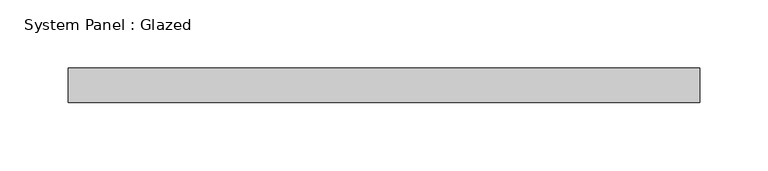
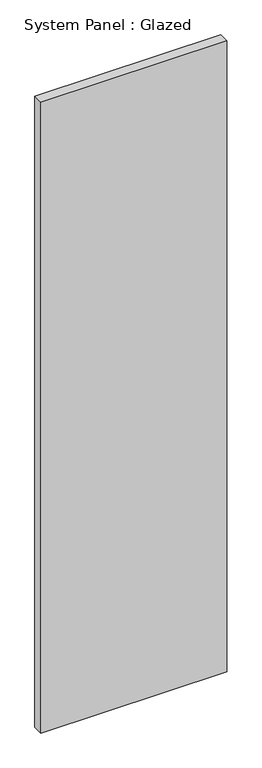
"""IFC4 building model written with IfcOpenShell, lengths in millimetres: plate geometry, System Panel : Glazed."""

from ifc_helpers import new_model, si_unit, origin, origin_with_axes, place, context, project, spatial, polyline, outline, extrude, source, transform, mapped, element, save


def system_panel_glazed_bb2283f1(model_context):
    return source(origin(), model_context, "Body", "SweptSolid", [
        extrude(outline(polyline([(231.775, 19.05), (-231.775, 19.05), (-231.775, 44.45), (231.775, 44.45), (231.775, 19.05)])), origin_with_axes(), (0.0, 0.0, 1.0), 1662.0304763),
    ])


if __name__ == "__main__":
    model = new_model("IFC4")
    model_context = context("Model", 3, world=origin())
    ifc_project = project(units=[si_unit("LENGTHUNIT", "METRE", prefix="MILLI")], contexts=[model_context])
    site = spatial("IfcSite", under=ifc_project)
    building = spatial("IfcBuilding", under=site)
    placement = place(None, origin())
    system_panel_glazed_shape = system_panel_glazed_bb2283f1(model_context)
    element("IfcPlate", 1, ObjectType="System Panel : Glazed", at=placement, inside=building, context=model_context, shape_type="MappedRepresentation", body=[
        mapped(system_panel_glazed_shape, transform((0.0, 0.0, 0.0), x_axis=(1.0, 0.0, 0.0), y_axis=(0.0, 1.0, 0.0), z_axis=(0.0, 0.0, 1.0))),
    ])
    save(model, "model.ifc")

# Revit data of these elements
# Type "System Panel : Glazed"
#   Construction Type Id = "GSP4R"
#   Analytic Construction = "1/8 in Pilkington single glazing"
#   Visual Light Transmittance = 0.9
#   Solar Heat Gain Coefficient = 0.86
#   Heat Transfer Coefficient (U) = 1.18115 BTU/(h·ft²·°F)
#   Define Thermal Properties by = 1
# Element 1 (IfcPlate, "System Panel : Glazed")
#   Materials on its faces: "Glass"
# Materials
#   "Glass": class "Glass", colour RGB 0 128 192, transparency 0.75, Description = "Soda Lime Glass", Cost = 0
